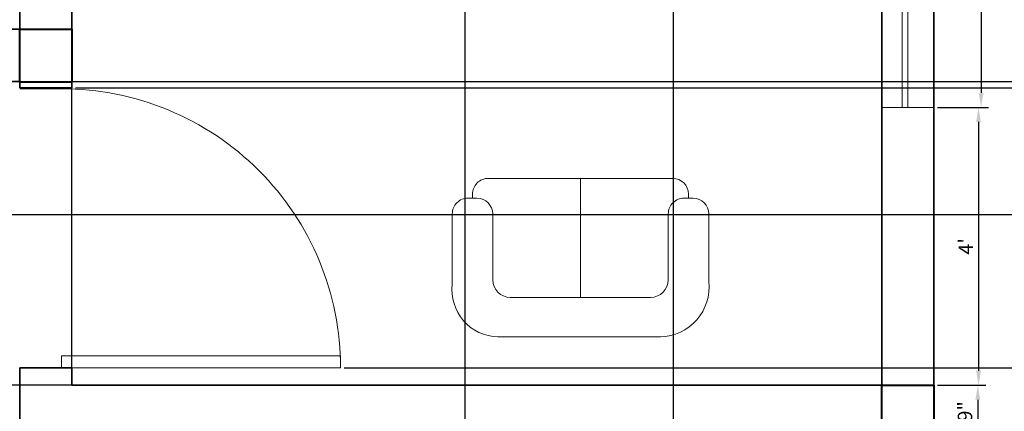
# Model space of a CAD drawing. Units: inches. Extents: x 1624 to 3956, y 1589 to 5028.
# Tile 11 of 16: x 1943 to 2113, y 2250 to 2317. Entities that reach past the tile are written whole.
import ezdxf

# ---------------------------------------------------------------- set-up
doc = ezdxf.new("R2010")
doc.units = ezdxf.units.IN
for name, color, linetype, lineweight in [('A-ANNO-DIMS', 2, 'Continuous', 13), ('A-COLS', 1, 'Continuous', 40), ('A-DOOR', 3, 'Continuous', 18), ('A-FURN', 8, 'Continuous', 18), ('A-GLAZ', 4, 'Continuous', 18), ('A-WALL', 7, 'Continuous', 35)]:
    doc.layers.add(name, color=color, linetype=linetype, lineweight=lineweight)
doc.styles.get("Standard").update_dxf_attribs({"font": 'arial.ttf'})
doc.dimstyles.new('Copy of ISO-25', dxfattribs={"dimtxt": 2.5, "dimasz": 2.5, "dimexe": 1.25, "dimexo": 0.625, "dimtad": 1, "dimdec": 1, "dimlunit": 4, "dimtxsty": 'Standard', "dimcen": 2.5, "dimadec": 0, "dimazin": 0, "dimtfac": 1, "dimtdec": 1, "dimtmove": 0, "dimatfit": 3, "dimfxl": 1, "dimarcsym": 0})

# ---------------------------------------------------------------- blocks, each defined once
blk = doc.blocks.new('*U5')
for p, q in [((0, 0), (0, 6)), ((40, 0), (40, 6))]:
    blk.add_line(p, q)
blk.add_lwpolyline([(0, 0), (0, -40), (1.75, -40), (1.75, 0)], close=True)
blk.add_arc((0, 0), 40, 270, 0)
blk = doc.blocks.new('A$C6D011943')
for p, q in [((1.4484, 1.0893), (0.3319, 1.0893)), ((1.3639, 0.8177), (0.3983, 0.8177)), ((0.8811, 0.8177), (0.8811, 0)), ((0, 0.7091), (0, 0.2474)), ((0.2776, 0.697), (0.2776, 0.2444)), ((1.4846, 0.2444), (1.4846, 0.697)), ((1.7622, 0.2474), (1.7622, 0.7272)), ((0.1086, 0.1358), (0.169, 0.1358)), ((0.1388, 0.1086), (0.1388, 0.1358)), ((1.5932, 0.1358), (1.6536, 0.1358)), ((1.6475, 0.1358), (1.6234, 0.1358)), ((1.6234, 0.1086), (1.6234, 0.1358)), ((1.5148, 0), (0.2474, 0))]:
    blk.add_line(p, q)
for centre, radius, start, end in [((0.3394, 0.7478), 0.3416, 91.2564, 186.501), ((1.4409, 0.7658), 0.3236, 353.159, 88.6697), ((0.3983, 0.697), 0.1207, 90, 180), ((1.3639, 0.697), 0.1207, 0, 90), ((0.1086, 0.2444), 0.1086, 180, 270), ((0.169, 0.2444), 0.1086, 270, 0.00001), ((1.5932, 0.2444), 0.1086, 180, 270), ((1.6536, 0.2444), 0.1086, 270, 0.00001), ((0.2474, 0.1086), 0.1086, 180, 270), ((1.5148, 0.1086), 0.1086, 270, 0)]:
    blk.add_arc(centre, radius, start, end)
blk = doc.blocks.new('*D36')
at = {"layer": 'A-ANNO-DIMS', "color": 0, "lineweight": -2, "transparency": 16777216}
for p, q in [((2101.2, 2374.29), (2109.99, 2374.29)), ((2108.74, 2371.79), (2108.74, 2304.79)), ((2101.2, 2302.29), (2109.99, 2302.29))]:
    blk.add_line(p, q, dxfattribs=at)
at = {"layer": 'A-ANNO-DIMS', "color": 0, "transparency": 16777216}
for points in [[(2108.33, 2371.79), (2109.16, 2371.79), (2108.74, 2374.29)], [(2108.33, 2304.79), (2109.16, 2304.79), (2108.74, 2302.29)]]:
    blk.add_solid(points, dxfattribs=at)
at = {"layer": 'Defpoints', "color": 0, "transparency": 16777216}
for p in [(2100.58, 2374.29), (2100.58, 2302.29), (2108.74, 2302.29)]:
    blk.add_point(p, dxfattribs=at)
at = {"layer": 'A-ANNO-DIMS', "color": 0, "transparency": 16777216, "insert": (2106.84, 2338.29), "char_height": 2.5, "attachment_point": 5, "rotation": 90}
blk.add_mtext("6'", dxfattribs=at)
blk = doc.blocks.new('*D37')
at = {"layer": 'A-ANNO-DIMS', "color": 0, "lineweight": -2, "transparency": 16777216}
for p, q in [((2101.2, 2302.29), (2109.54, 2302.29)), ((2108.29, 2299.79), (2108.29, 2256.79)), ((2101.2, 2254.29), (2109.54, 2254.29))]:
    blk.add_line(p, q, dxfattribs=at)
at = {"layer": 'A-ANNO-DIMS', "color": 0, "transparency": 16777216}
for points in [[(2107.88, 2299.79), (2108.71, 2299.79), (2108.29, 2302.29)], [(2107.88, 2256.79), (2108.71, 2256.79), (2108.29, 2254.29)]]:
    blk.add_solid(points, dxfattribs=at)
at = {"layer": 'Defpoints', "color": 0, "transparency": 16777216}
for p in [(2100.58, 2302.29), (2100.58, 2254.29), (2108.29, 2254.29)]:
    blk.add_point(p, dxfattribs=at)
at = {"layer": 'A-ANNO-DIMS', "color": 0, "transparency": 16777216, "insert": (2106.42, 2278.29), "char_height": 2.5, "attachment_point": 5, "rotation": 90}
blk.add_mtext("4'", dxfattribs=at)
blk = doc.blocks.new('*D38')
at = {"layer": 'A-ANNO-DIMS', "color": 0, "lineweight": -2, "transparency": 16777216}
for p, q in [((2101.2, 2254.29), (2109.43, 2254.29)), ((2108.18, 2251.79), (2108.18, 2247.79)), ((2101.2, 2245.29), (2109.43, 2245.29))]:
    blk.add_line(p, q, dxfattribs=at)
at = {"layer": 'A-ANNO-DIMS', "color": 0, "transparency": 16777216}
for points in [[(2107.76, 2251.79), (2108.59, 2251.79), (2108.18, 2254.29)], [(2107.76, 2247.79), (2108.59, 2247.79), (2108.18, 2245.29)]]:
    blk.add_solid(points, dxfattribs=at)
at = {"layer": 'Defpoints', "color": 0, "transparency": 16777216}
for p in [(2100.58, 2254.29), (2100.58, 2245.29), (2108.18, 2245.29)]:
    blk.add_point(p, dxfattribs=at)
at = {"layer": 'A-ANNO-DIMS', "color": 0, "transparency": 16777216, "insert": (2106.28, 2249.79), "char_height": 2.5, "attachment_point": 5, "rotation": 90}
blk.add_mtext('9"', dxfattribs=at)
blk = doc.blocks.new('COLUMN-9x9')
for p, q in [((0, 0), (0, 9)), ((0, 9), (9, 9)), ((9, 9), (9, 0)), ((9, 0), (0, 0))]:
    blk.add_line(p, q)
blk = doc.blocks.new('WINDOW-72IN')
for p, q in [((0, 9), (0, 0)), ((72, 0), (72, 9)), ((0, 4.5), (72, 4.5)), ((0, 3.5), (72, 3.5))]:
    blk.add_line(p, q)
blk = doc.blocks.new('*D79')
at = {"layer": 'A-ANNO-DIMS', "color": 0, "lineweight": -2, "transparency": 16777216}
for p, q in [((2090.95, 2422.29), (1628.86, 2422.29)), ((1630.11, 2419.79), (1630.11, 2256.79)), ((2090.95, 2254.29), (1628.86, 2254.29))]:
    blk.add_line(p, q, dxfattribs=at)
at = {"layer": 'A-ANNO-DIMS', "color": 0, "transparency": 16777216}
for points in [[(1629.69, 2419.79), (1630.53, 2419.79), (1630.11, 2422.29)], [(1629.69, 2256.79), (1630.53, 2256.79), (1630.11, 2254.29)]]:
    blk.add_solid(points, dxfattribs=at)
at = {"layer": 'Defpoints', "color": 0, "transparency": 16777216}
for p in [(2091.58, 2422.29), (1630.11, 2254.29), (2091.58, 2254.29)]:
    blk.add_point(p, dxfattribs=at)
at = {"layer": 'A-ANNO-DIMS', "color": 0, "transparency": 16777216, "insert": (1628.21, 2338.29), "char_height": 2.5, "attachment_point": 5, "rotation": 90}
blk.add_mtext('14\'-0"', dxfattribs=at)
blk = doc.blocks.new('*D81')
at = {"layer": 'A-ANNO-DIMS', "color": 0, "lineweight": -2, "transparency": 16777216}
for p, q in [((1951.58, 2254.92), (1951.58, 2612.84)), ((2091.58, 2254.92), (2091.58, 2612.84)), ((1954.08, 2611.59), (2089.08, 2611.59))]:
    blk.add_line(p, q, dxfattribs=at)
at = {"layer": 'A-ANNO-DIMS', "color": 0, "transparency": 16777216}
for points in [[(1954.08, 2612.01), (1954.08, 2611.18), (1951.58, 2611.59)], [(2089.08, 2612.01), (2089.08, 2611.18), (2091.58, 2611.59)]]:
    blk.add_solid(points, dxfattribs=at)
at = {"layer": 'Defpoints', "color": 0, "transparency": 16777216}
for p in [(2091.58, 2611.59), (1951.58, 2254.29), (2091.58, 2254.29)]:
    blk.add_point(p, dxfattribs=at)
at = {"layer": 'A-ANNO-DIMS', "color": 0, "transparency": 16777216, "insert": (2021.58, 2613.5), "char_height": 2.5, "attachment_point": 5}
blk.add_mtext('11\'-8"', dxfattribs=at)
blk = doc.blocks.new('*D90')
at = {"layer": 'A-ANNO-DIMS', "color": 0, "lineweight": -2, "transparency": 16777216}
for p, q in [((2019.58, 1941.92), (2019.58, 2612.84)), ((2055.58, 1941.92), (2055.58, 2612.84)), ((2022.08, 2611.59), (2053.08, 2611.59))]:
    blk.add_line(p, q, dxfattribs=at)
at = {"layer": 'A-ANNO-DIMS', "color": 0, "transparency": 16777216}
for points in [[(2022.08, 2612.01), (2022.08, 2611.18), (2019.58, 2611.59)], [(2053.08, 2612.01), (2053.08, 2611.18), (2055.58, 2611.59)]]:
    blk.add_solid(points, dxfattribs=at)
at = {"layer": 'Defpoints', "color": 0, "transparency": 16777216}
for p in [(2055.58, 2611.59), (2019.58, 1941.29), (2055.58, 1941.29)]:
    blk.add_point(p, dxfattribs=at)
at = {"layer": 'A-ANNO-DIMS', "color": 0, "transparency": 16777216, "insert": (2037.58, 2613.5), "char_height": 2.5, "attachment_point": 5}
blk.add_mtext('3\'-0"', dxfattribs=at)
blk = doc.blocks.new('*D96')
at = {"layer": 'A-ANNO-DIMS', "color": 0, "lineweight": -2, "transparency": 16777216}
for p, q in [((1952.2, 2305.65), (2217.63, 2305.65)), ((2216.38, 2303.15), (2216.38, 2259.79)), ((1998.67, 2257.29), (2217.63, 2257.29))]:
    blk.add_line(p, q, dxfattribs=at)
at = {"layer": 'A-ANNO-DIMS', "color": 0, "transparency": 16777216}
for points in [[(2215.96, 2303.15), (2216.8, 2303.15), (2216.38, 2305.65)], [(2215.96, 2259.79), (2216.8, 2259.79), (2216.38, 2257.29)]]:
    blk.add_solid(points, dxfattribs=at)
at = {"layer": 'Defpoints', "color": 0, "transparency": 16777216}
for p in [(1951.58, 2305.65), (1998.04, 2257.29), (2216.38, 2257.29)]:
    blk.add_point(p, dxfattribs=at)
at = {"layer": 'A-ANNO-DIMS', "color": 0, "transparency": 16777216, "insert": (2214.46, 2281.47), "char_height": 2.5, "attachment_point": 5, "rotation": 90}
blk.add_mtext('4\'-0 1/2"', dxfattribs=at)
blk = doc.blocks.new('*D100')
at = {"layer": 'A-ANNO-DIMS', "color": 0, "lineweight": -2, "transparency": 16777216}
for p, q in [((1738.2, 2306.79), (2217.63, 2306.79)), ((2216.38, 2286.28), (2216.38, 2304.29)), ((1761.2, 2283.78), (2217.63, 2283.78))]:
    blk.add_line(p, q, dxfattribs=at)
at = {"layer": 'A-ANNO-DIMS', "color": 0, "transparency": 16777216}
for points in [[(2215.96, 2304.29), (2216.8, 2304.29), (2216.38, 2306.79)], [(2215.96, 2286.28), (2216.8, 2286.28), (2216.38, 2283.78)]]:
    blk.add_solid(points, dxfattribs=at)
at = {"layer": 'Defpoints', "color": 0, "transparency": 16777216}
for p in [(1737.58, 2306.79), (2216.38, 2306.79), (1760.58, 2283.78)]:
    blk.add_point(p, dxfattribs=at)
at = {"layer": 'A-ANNO-DIMS', "color": 0, "transparency": 16777216, "insert": (2214.5, 2295.29), "char_height": 2.5, "attachment_point": 5, "rotation": 90}
blk.add_mtext('1\'-11"', dxfattribs=at)

msp = doc.modelspace()

# ---------------------------------------------------------------- linework, layer by layer
at = {"layer": 'A-COLS'}
for p, q in [((1942.58, 2315.79), (1951.58, 2315.79)), ((1942.58, 2306.65), (1942.58, 2315.79)), ((1951.58, 2315.79), (1951.58, 2306.65)), ((1951.58, 2306.65), (1942.58, 2306.65))]:
    msp.add_line(p, q, dxfattribs=at)
at = {"layer": 'A-GLAZ'}
msp.add_line((2100.58, 2374.29), (2100.58, 2302.29), dxfattribs=at)
at = {"layer": 'A-WALL'}
for p, q in [((1942.58, 2315.79), (1942.58, 2432.79)), ((1951.58, 2305.65), (1951.58, 2422.29)), ((2091.58, 2422.29), (2091.58, 2254.29)), ((2100.58, 2374.29), (2100.58, 2254.29)), ((1942.58, 2315.79), (1929.52, 2315.79)), ((1929.52, 2315.79), (1942.58, 2315.79)), ((1929.52, 2306.79), (1942.58, 2306.79)), ((1942.58, 2305.65), (1942.58, 2306.79)), ((1951.58, 2306.65), (1951.58, 2305.65)), ((1951.58, 2305.65), (1942.58, 2305.65)), ((1942.58, 2254.29), (1942.58, 2257.29)), ((1951.58, 2257.29), (1942.58, 2257.29)), ((1951.58, 2254.29), (1951.58, 2257.29)), ((1951.58, 2254.29), (1951.58, 2257.29)), ((1942.58, 2245.29), (1942.58, 2254.29)), ((1960.58, 2254.29), (1951.58, 2254.29)), ((2091.58, 2254.29), (1960.58, 2254.29)), ((2100.58, 2254.29), (2100.58, 2161.29)), ((2100.58, 2245.29), (2100.58, 2254.29))]:
    msp.add_line(p, q, dxfattribs=at)

# ---------------------------------------------------------------- block references
at = {"layer": 'A-COLS', "rotation": 270.0000000000029}
msp.add_blockref('COLUMN-9x9', (2091.58, 2254.29), dxfattribs=at)
at = {"layer": 'A-DOOR', "xscale": 1.205774439306444, "yscale": 1.205774439306444, "zscale": 1.205774439306444, "rotation": 89.99999999999999}
msp.add_blockref('*U5', (1949.81, 2257.29), dxfattribs=at)
at = {"layer": 'A-FURN', "xscale": 25.14761962403201, "yscale": 25.14761962403201, "zscale": 25.14761962403201, "rotation": 180}
msp.add_blockref('A$C6D011943', (2061.66, 2290.04), dxfattribs=at)
at = {"layer": 'A-GLAZ', "rotation": 270}
msp.add_blockref('WINDOW-72IN', (2091.58, 2374.29), dxfattribs=at)

# ---------------------------------------------------------------- dimensions: what is measured, and where the dimension line sits
at = {"layer": 'A-ANNO-DIMS'}
for base, p1, p2, picture, middle in [((2091.58, 2611.59), (1951.58, 2254.29), (2091.58, 2254.29), '*D81', (2021.58, 2613.5)), ((2055.58, 2611.59), (2019.58, 1941.29), (2055.58, 1941.29), '*D90', (2037.58, 2613.5))]:
    dim = msp.add_linear_dim(base=base, p1=p1, p2=p2, dimstyle='Copy of ISO-25', override={"dimdec": 1, "dimlfac": 1, "dimrnd": 0, "dimzin": 1, "dimdsep": 46, "dimlunit": 4, "dimfrac": 2}, dxfattribs=at)
    dim.commit()
    dim.dimension.update_dxf_attribs({"geometry": picture, "text_midpoint": middle})
for base, p1, p2, override, picture, middle in [((1630.11, 2254.29), (2091.58, 2422.29), (2091.58, 2254.29), {"dimdec": 1, "dimlfac": 1, "dimrnd": 0, "dimzin": 1, "dimdsep": 46, "dimlunit": 4, "dimfrac": 2}, '*D79', (1628.21, 2338.29)), ((2108.74, 2302.29), (2100.58, 2374.29), (2100.58, 2302.29), {"dimclrd": 0, "dimclre": 0, "dimclrt": 0}, '*D36', (2106.84, 2338.29)), ((2216.38, 2306.79), (1760.58, 2283.78), (1737.58, 2306.79), {"dimdec": 1, "dimlfac": 1, "dimrnd": 0, "dimzin": 1, "dimdsep": 46, "dimlunit": 4, "dimfrac": 2}, '*D100', (2214.5, 2295.29)), ((2216.38, 2257.29), (1951.58, 2305.65), (1998.04, 2257.29), {"dimdec": 1, "dimlfac": 1, "dimrnd": 0, "dimzin": 1, "dimdsep": 46, "dimlunit": 4, "dimfrac": 2}, '*D96', (2214.46, 2281.47)), ((2108.29, 2254.29), (2100.58, 2302.29), (2100.58, 2254.29), {"dimclrd": 0, "dimclre": 0, "dimclrt": 0}, '*D37', (2106.42, 2278.29)), ((2108.18, 2245.29), (2100.58, 2254.29), (2100.58, 2245.29), {"dimclrd": 0, "dimclre": 0, "dimclrt": 0}, '*D38', (2106.28, 2249.79))]:
    dim = msp.add_linear_dim(base=base, p1=p1, p2=p2, angle=90, dimstyle='Copy of ISO-25', override=override, dxfattribs=at)
    dim.commit()
    dim.dimension.update_dxf_attribs({"geometry": picture, "text_midpoint": middle})

doc.saveas('drawing.dxf')
